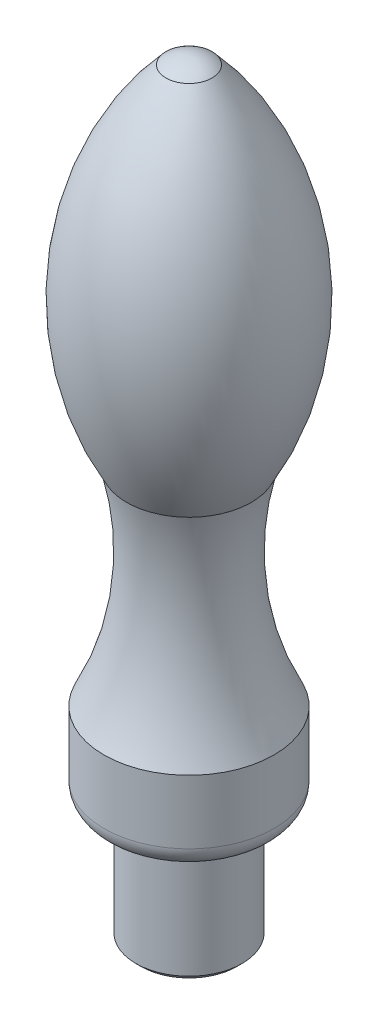
from build123d import *

# Parameters (mm, degrees)
SHANK_SKETCH_10_R          = 5
SHANK_10_DEPTH             = 11
SHANK_END_CHAMFER_0_5_SIZE = 0.5
COLLAR_SKETCH_16_R         = 8
COLLAR_16_DEPTH            = 8
COLLAR_FILLET_R2_R         = 2


with BuildPart() as part:
    # Shank Sketch Ø10 → Shank Ø10 (new body)
    with BuildSketch(Plane(origin=(0, 0, 0), x_dir=(1, 0, 0), z_dir=(0, 1, 0))):
        with Locations(Location((0, 0, 0), (0, 0, 270))):
            Circle(SHANK_SKETCH_10_R)
    extrude(amount=SHANK_10_DEPTH)

    # Shank End Chamfer 0.5
    shank_end_chamfer_0_5_edges = [part.edges().sort_by_distance(p)[0] for p in [
        (0, 0, -5),
    ]]
    chamfer(shank_end_chamfer_0_5_edges, length=SHANK_END_CHAMFER_0_5_SIZE)

    # Collar Sketch Ø16 → Collar Ø16 (add)
    with BuildSketch(Plane(origin=(0, 11, 0), x_dir=(1, 0, 0), z_dir=(0, 1, 0))):
        with Locations(Location((0, 0, 0), (0, 0, 270))):
            Circle(COLLAR_SKETCH_16_R)
    extrude(amount=COLLAR_16_DEPTH)

    # Collar Fillet R2
    collar_fillet_r2_edges = [part.edges().sort_by_distance(p)[0] for p in [
        (0, 11, -8),
    ]]
    fillet(collar_fillet_r2_edges, radius=COLLAR_FILLET_R2_R)

    # Grip Profile Sketch → Grip Knob (revolve)
    with BuildSketch(Plane.XY, mode=Mode.PRIVATE) as grip_knob_sk:
        with BuildLine():
            Line((-8, 19), (0, 19))
            Line((0, 19), (0, 72))
            ThreePointArc((0, 72), (-1.143202963, 71.811669668), (-2.165583383, 71.266582881))
            ThreePointArc((-2.165583383, 71.266582881), (-9.343191716, 55.495909404), (-5.86603911, 38.521174854))
            ThreePointArc((-5.86603911, 38.521174854), (-5.165533535, 28.567374361), (-8, 19))
        make_face()
    revolve(grip_knob_sk.sketch.rotate(Axis((0, 0, 0), (0, 1, 0)), 270), axis=Axis((0, 0, 0), (0, 1, 0)))


solid = part.part
